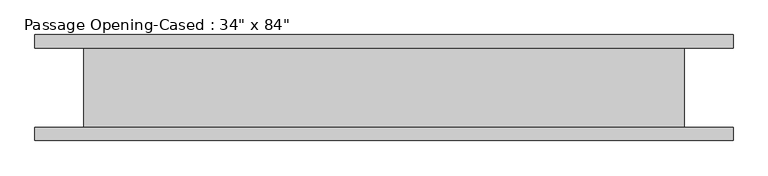
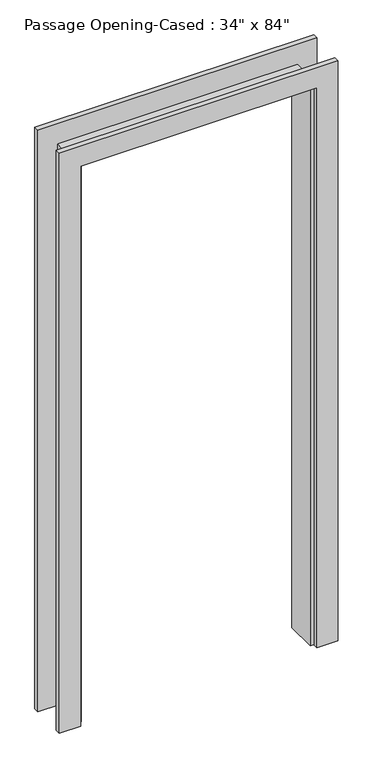
"""IFC4 building model written with IfcOpenShell, lengths in millimetres: proxy geometry."""

from ifc_helpers import new_model, si_unit, frame, origin, place, context, project, spatial, polyline, outline, extrude, faceted_brep, source, transform, mapped, element, save


def proxy_dc468f74(model_context):
    return source(origin(), model_context, "Body", "SolidModel", [
        faceted_brep([(404.5613433, 57.15, 0.0), (423.6113433, 57.15, 0.0), (423.6113433, -57.15, 0.0), (404.5613433, -57.15, 0.0), (404.5613433, 57.15, 2114.55), (423.6113433, 57.15, 2133.6), (423.6113433, -57.15, 2133.6), (404.5613433, -57.15, 2114.55), (-420.9386567, 57.15, 2114.55), (-439.9886567, 57.15, 2133.6), (-439.9886567, -57.15, 2133.6), (-420.9386567, -57.15, 2114.55), (-420.9386567, 57.15, 0.0), (-420.9386567, -57.15, 0.0), (-439.9886567, -57.15, 0.0), (-439.9886567, 57.15, 0.0)], [[[0, 1, 2, 3]], [[1, 0, 4, 5]], [[2, 1, 5, 6]], [[3, 2, 6, 7]], [[0, 3, 7, 4]], [[5, 4, 8, 9]], [[6, 5, 9, 10]], [[7, 6, 10, 11]], [[4, 7, 11, 8]], [[12, 13, 14, 15]], [[9, 8, 12, 15]], [[10, 9, 15, 14]], [[11, 10, 14, 13]], [[8, 11, 13, 12]]]),
        extrude(outline(polyline([(0.0, 493.4613433), (2209.8, 493.4613433), (2209.8, -509.8386567), (0.0, -509.8386567), (0.0, -433.6386567), (2127.25, -433.6386567), (2127.25, 417.2613433), (0.0, 417.2613433), (0.0, 493.4613433)])), frame((0.0, 57.15, 0.0), z_axis=(0.0, 1.0, 0.0), x_axis=(0.0, 0.0, 1.0)), (0.0, 0.0, 1.0), 19.05),
        extrude(outline(polyline([(0.0, -433.6386567), (2127.25, -433.6386567), (2127.25, 417.2613433), (0.0, 417.2613433), (0.0, 493.4613433), (2203.45, 493.4613433), (2203.45, -509.8386567), (0.0, -509.8386567), (0.0, -433.6386567)])), frame((0.0, -76.2, 0.0), z_axis=(0.0, 1.0, 0.0), x_axis=(0.0, 0.0, 1.0)), (0.0, 0.0, 1.0), 19.05),
    ])


if __name__ == "__main__":
    model = new_model("IFC4")
    model_context = context("Model", 3, world=origin())
    ifc_project = project(units=[si_unit("LENGTHUNIT", "METRE", prefix="MILLI")], contexts=[model_context])
    site = spatial("IfcSite", under=ifc_project)
    building = spatial("IfcBuilding", under=site)
    placement = place(None, origin())
    proxy_shape = proxy_dc468f74(model_context)
    element("IfcBuildingElementProxy", 1, Name="Passage Opening-Cased : 34\" x 84\"", ObjectType="Passage Opening-Cased : 34\" x 84\"", at=placement, inside=building, context=model_context, shape_type="MappedRepresentation", body=[
        mapped(proxy_shape, transform((0.0, 0.0, 0.0), x_axis=(1.0, 0.0, 0.0), y_axis=(0.0, 1.0, 0.0), z_axis=(0.0, 0.0, 1.0))),
    ])
    save(model, "model.ifc")

# Revit data of these elements
# Type "Passage Opening-Cased : 34\" x 84\""
#   Height = 7' - 0"
#   Trim Thickness = 0' - 0 3/4"
#   Trim Width = 0' - 3"
#   Width = 2' - 10"
#   Frame Material = Door - Frame
#   Default Elevation = 0
# Element 1 (IfcBuildingElementProxy, "Passage Opening-Cased : 34\" x 84\"")
#   Materials on its faces: "Door - Frame"
# Materials
#   "Door - Frame": colour RGB 118 70 51, transparency 0, Cost = 0
